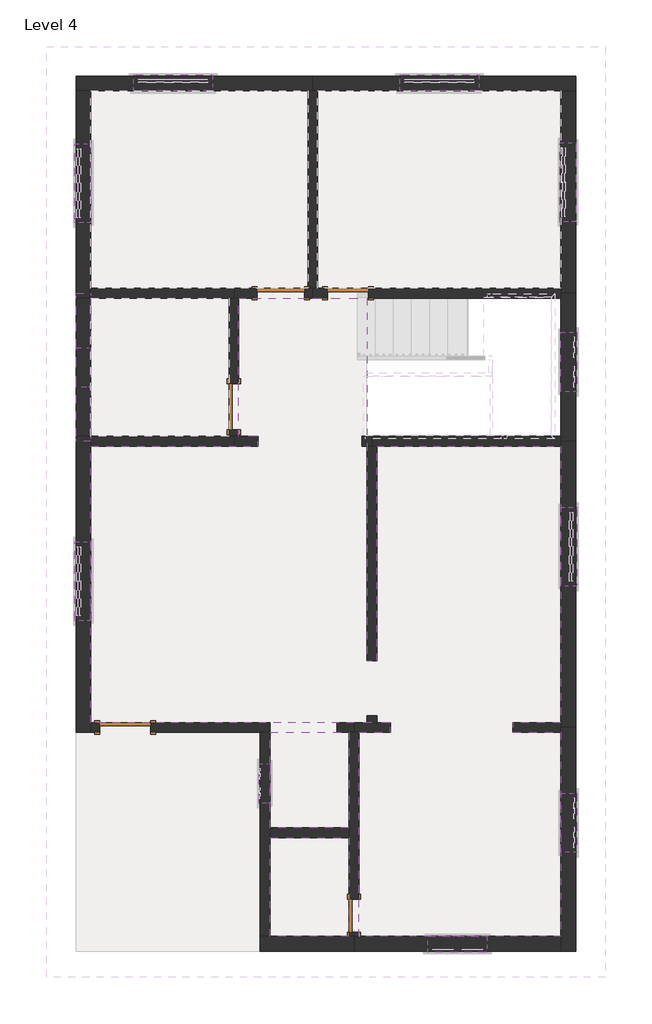
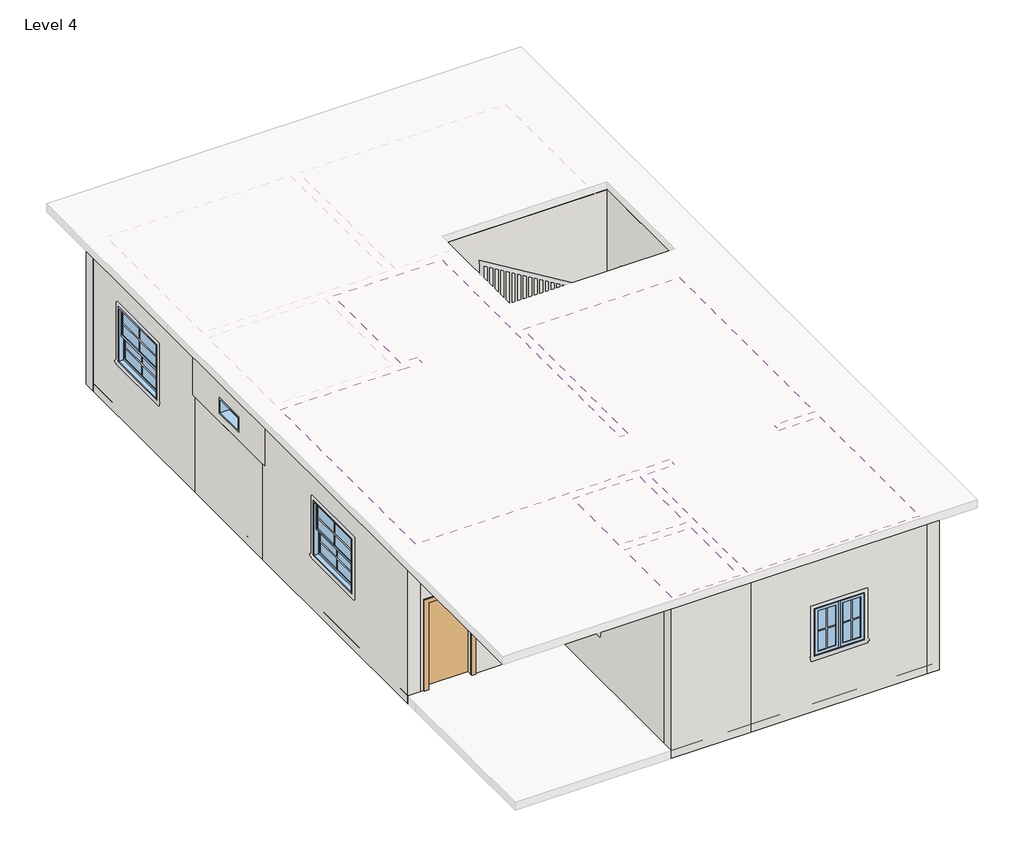
# One storey, part 1 of 2: 26 walls, 11 windows, 5 doors, 3 coverings.
"""IFC4 building model written with IfcOpenShell, lengths in millimetres."""

from ifc_helpers import new_model, si_unit, frame, origin, place, context, project, spatial, polyline, circle_curve, outline, extrude, faceted_brep, transform, mapped, element, save
from ifc_brep_helpers import plane_surface, revolved_surface, advanced_brep
from components import door_85c31a06, door_fe267433, door_77f51d0b, door_a6948854, door_ee35e093, fixed_2_8c8825d0, window_casement_double_2_fb285ced, window_casement_double_3_90de19e9, window_double_hung_4_eadb0177, window_double_hung_4_aab3aae7

model = new_model("IFC4")

# Units and contexts
model_context = context("Model", 3, world=origin())
ifc_project = project(units=[si_unit("LENGTHUNIT", "METRE", prefix="MILLI")], contexts=[model_context])

# Site, building, storey
site = spatial("IfcSite", under=ifc_project)
building = spatial("IfcBuilding", under=site)
storey = spatial("IfcBuildingStorey", under=building, Name="Level 4", Elevation=9601.2)

# Coverings
placement = place(None, origin())
element("IfcCovering", 1, ObjectType="2' x 4' ACT System", at=placement, inside=storey, context=model_context, shape_type="SweptSolid", body=[
    extrude(outline(polyline([(1592.635938, -3451.4142637), (1592.635938, -6601.0142637), (-1531.564062, -6601.0142637), (-1531.564062, -3451.4142637), (-1042.9877715, -3451.4142637), (-1042.9877715, -3299.0142637), (-1607.764062, -3299.0142637), (-5671.764062, -3299.0142637), (-5671.764062, 968.1857363), (-3538.164062, 968.1857363), (-3088.5741654, 968.1857363), (-3088.5741654, 1120.5857363), (-3385.764062, 1120.5857363), (-3385.764062, 3254.1857363), (-2242.764062, 3254.1857363), (-1404.564062, 3254.1857363), (-1404.564062, -2346.4297845), (-1252.164062, -2346.4297845), (-1252.164062, 968.1857363), (1592.635938, 968.1857363), (1592.635938, -3299.0142637), (852.655246, -3299.0142637), (852.655246, -3451.4142637), (1592.635938, -3451.4142637)])), frame((0.0, 0.0, 12649.2), z_axis=(0.0, 0.0, 1.0), x_axis=(1.0, 0.0, 0.0)), (0.0, 0.0, 1.0), 57.15),
])
element("IfcCovering", 2, ObjectType="2' x 4' ACT System", at=placement, inside=storey, context=model_context, shape_type="SweptSolid", body=[
    extrude(outline(polyline([(-2903.164062, -4924.6142637), (-2903.164062, -3451.4142637), (-1683.964062, -3451.4142637), (-1683.964062, -4924.6142637), (-2903.164062, -4924.6142637)])), frame((0.0, 0.0, 12649.2), z_axis=(0.0, 0.0, 1.0), x_axis=(1.0, 0.0, 0.0)), (0.0, 0.0, 1.0), 57.15),
])
element("IfcCovering", 3, ObjectType="2' x 4' ACT System", at=placement, inside=storey, context=model_context, shape_type="SweptSolid", body=[
    extrude(outline(polyline([(-2903.164062, -6601.0142637), (-2903.164062, -5077.0142637), (-1683.964062, -5077.0142637), (-1683.964062, -6601.0142637), (-2903.164062, -6601.0142637)])), frame((0.0, 0.0, 12649.2), z_axis=(0.0, 0.0, 1.0), x_axis=(1.0, 0.0, 0.0)), (0.0, 0.0, 1.0), 57.15),
])

# Doors
door_shape = door_85c31a06(model_context)
element("IfcDoor", 4, ObjectType="Single-Flush : 1'8\"", at=placement, inside=storey, context=model_context, shape_type="MappedRepresentation", body=[
    mapped(door_shape, transform((-1607.764062, -6283.5142637, 9753.6), x_axis=(0.0, -1.0, 0.0), y_axis=(1.0, 0.0, 0.0), z_axis=(0.0, 0.0, 1.0))),
])
door_2_shape = door_fe267433(model_context)
element("IfcDoor", 5, ObjectType="Single-Flush : 2'1\"", at=placement, inside=storey, context=model_context, shape_type="MappedRepresentation", body=[
    mapped(door_2_shape, transform((-1696.664062, 3330.3857363, 9753.6), x_axis=(-1.0, 0.0, 0.0), y_axis=(0.0, -1.0, 0.0), z_axis=(0.0, 0.0, 1.0))),
])
door_3_shape = door_77f51d0b(model_context)
element("IfcDoor", 6, ObjectType="Single-Flush : 2'4\"", at=placement, inside=storey, context=model_context, shape_type="MappedRepresentation", body=[
    mapped(door_3_shape, transform((-3461.964062, 1577.7857363, 9753.6), x_axis=(0.0, -1.0, 0.0), y_axis=(1.0, 0.0, 0.0), z_axis=(0.0, 0.0, 1.0))),
])
door_4_shape = door_a6948854(model_context)
element("IfcDoor", 7, ObjectType="Single-Flush : 2'5\"", at=placement, inside=storey, context=model_context, shape_type="MappedRepresentation", body=[
    mapped(door_4_shape, transform((-2738.064062, 3330.3857363, 9753.6), x_axis=(1.0, 0.0, 0.0), y_axis=(0.0, 1.0, 0.0), z_axis=(0.0, 0.0, 1.0))),
])
door_5_shape = door_ee35e093(model_context)
element("IfcDoor", 8, ObjectType="Single-Flush : 2'7\"", at=placement, inside=storey, context=model_context, shape_type="MappedRepresentation", body=[
    mapped(door_5_shape, transform((-5144.714062, -3375.2142637, 9753.6), x_axis=(-1.0, 0.0, 0.0), y_axis=(0.0, -1.0, 0.0), z_axis=(0.0, 0.0, 1.0))),
])

# Walls
element("IfcWall", 9, ObjectType="Generic - 6\"", at=placement, inside=storey, context=model_context, shape_type="Brep", body=[
    faceted_brep([(-2318.964062, 6454.5857363, 9753.6), (-2318.964062, 3406.5857363, 9753.6), (-2318.964062, 3406.5857363, 12954.0), (-2318.964062, 6454.5857363, 12954.0), (-2166.564062, 6454.5857363, 9753.6), (-2166.564062, 6454.5857363, 12954.0), (-2166.564062, 3406.5857363, 12954.0), (-2166.564062, 3406.5857363, 9753.6), (-2242.764062, 6454.5857363, 9753.6), (-2242.764062, 3406.5857363, 9753.6), (-2242.764062, 3406.5857363, 12954.0), (-2242.764062, 6454.5857363, 12954.0)], [[[0, 1, 2, 3]], [[4, 5, 6, 7]], [[1, 0, 8, 4, 7, 9]], [[3, 2, 10, 6, 5, 11]], [[0, 3, 11, 5, 4, 8]], [[2, 1, 9, 7, 6, 10]]]),
])
element("IfcWall", 10, ObjectType="Generic - 6\"", at=placement, inside=storey, context=model_context, shape_type="Brep", body=[
    faceted_brep([(-5671.764062, 3254.1857363, 12954.0), (-5671.764062, 3254.1857363, 11582.4), (-5671.764062, 3254.1857363, 9753.6), (-3538.164062, 3254.1857363, 9753.6), (-3461.964062, 3254.1857363, 9753.6), (-3461.964062, 3254.1857363, 12954.0), (-3538.164062, 3254.1857363, 12954.0), (-5671.764062, 3406.5857363, 9753.6), (-5671.764062, 3406.5857363, 12954.0), (-3461.964062, 3406.5857363, 12954.0), (-3461.964062, 3406.5857363, 9753.6), (-5671.764062, 3330.3857363, 12954.0)], [[[0, 1, 2, 3, 4, 5, 6]], [[7, 8, 9, 10]], [[4, 3, 2, 7, 10]], [[5, 4, 10, 9]], [[0, 6, 5, 9, 8, 11]], [[0, 11, 8, 7, 2, 1]]]),
])
element("IfcWall", 11, ObjectType="Generic - 6\"", at=placement, inside=storey, context=model_context, shape_type="Brep", body=[
    faceted_brep([(-5671.764062, 968.1857363, 12954.0), (-5671.764062, 968.1857363, 9753.6), (-3461.964062, 968.1857363, 9753.6), (-3461.964062, 968.1857363, 12954.0), (-5671.764062, 1120.5857363, 9753.6), (-5671.764062, 1120.5857363, 11582.4), (-5671.764062, 1120.5857363, 12954.0), (-3538.164062, 1120.5857363, 12954.0), (-3461.964062, 1120.5857363, 12954.0), (-3461.964062, 1120.5857363, 9753.6), (-3538.164062, 1120.5857363, 9753.6), (-5671.764062, 1044.3857363, 12954.0)], [[[0, 1, 2, 3]], [[4, 5, 6, 7, 8, 9, 10]], [[2, 1, 4, 10, 9]], [[3, 2, 9, 8]], [[0, 3, 8, 7, 6, 11]], [[0, 11, 6, 5, 4, 1]]]),
])
element("IfcWall", 12, ObjectType="Generic - 6\"", at=placement, inside=storey, context=model_context, shape_type="Brep", body=[
    faceted_brep([(-1404.564062, 968.1857363, 9753.6), (-1404.564062, -2346.4297845, 9753.6), (-1404.564062, -2346.4297845, 12217.4), (-1404.564062, -3197.4142637, 12217.4), (-1404.564062, -3197.4142637, 12039.6), (-1404.564062, -3197.4142637, 9753.6), (-1404.564062, -3299.0142637, 9753.6), (-1404.564062, -3299.0142637, 12954.0), (-1404.564062, 968.1857363, 12954.0), (-1252.164062, -2346.4297845, 9753.6), (-1252.164062, 968.1857363, 9753.6), (-1252.164062, 968.1857363, 12954.0), (-1252.164062, -3299.0142637, 12954.0), (-1252.164062, -3299.0142637, 9753.6), (-1252.164062, -3197.4142637, 9753.6), (-1252.164062, -3197.4142637, 12039.6), (-1252.164062, -3197.4142637, 12217.4), (-1252.164062, -2346.4297845, 12217.4), (-1328.364062, 968.1857363, 9753.6), (-1328.364062, 968.1857363, 12954.0)], [[[0, 1, 2, 3, 4, 5, 6, 7, 8]], [[9, 10, 11, 12, 13, 14, 15, 16, 17]], [[7, 6, 13, 12]], [[1, 0, 18, 10, 9]], [[8, 7, 12, 11, 19]], [[2, 1, 9, 17]], [[3, 2, 17, 16]], [[3, 16, 15, 14, 5, 4]], [[6, 5, 14, 13]], [[0, 8, 19, 11, 10, 18]]]),
])
element("IfcWall", 13, ObjectType="Generic - 6\"", at=placement, inside=storey, context=model_context, shape_type="Brep", body=[
    faceted_brep([(-2903.164062, -3451.4142637, 12039.6), (-1865.8319448, -3451.4142637, 12039.6), (-1865.8319448, -3451.4142637, 9753.6), (-1683.964062, -3451.4142637, 9753.6), (-1607.764062, -3451.4142637, 9753.6), (-1607.764062, -3451.4142637, 12954.0), (-1683.964062, -3451.4142637, 12954.0), (-2903.164062, -3451.4142637, 12954.0), (-3055.564062, -3451.4142637, 12954.0), (-5671.764062, -3451.4142637, 12954.0), (-5671.764062, -3451.4142637, 9753.6), (-5538.414062, -3451.4142637, 9753.6), (-5538.414062, -3451.4142637, 11582.4), (-4751.014062, -3451.4142637, 11582.4), (-4751.014062, -3451.4142637, 9753.6), (-3055.564062, -3451.4142637, 9753.6), (-2903.164062, -3451.4142637, 9753.6), (-1865.8319448, -3299.0142637, 12039.6), (-2903.164062, -3299.0142637, 12039.6), (-2903.164062, -3299.0142637, 9753.6), (-4751.014062, -3299.0142637, 9753.6), (-4751.014062, -3299.0142637, 11582.4), (-5538.414062, -3299.0142637, 11582.4), (-5538.414062, -3299.0142637, 9753.6), (-5671.764062, -3299.0142637, 9753.6), (-5671.764062, -3299.0142637, 12954.0), (-1607.764062, -3299.0142637, 12954.0), (-1607.764062, -3299.0142637, 9753.6), (-1865.8319448, -3299.0142637, 9753.6)], [[[0, 1, 2, 3, 4, 5, 6, 7, 8, 9, 10, 11, 12, 13, 14, 15, 16]], [[17, 18, 19, 20, 21, 22, 23, 24, 25, 26, 27, 28]], [[17, 1, 0, 18]], [[1, 17, 28, 2]], [[22, 12, 11, 23]], [[12, 22, 21, 13]], [[13, 21, 20, 14]], [[10, 24, 23, 11]], [[27, 4, 3, 2, 28]], [[19, 16, 15, 14, 20]], [[5, 4, 27, 26]], [[9, 8, 7, 6, 5, 26, 25]], [[10, 9, 25, 24]], [[18, 0, 16, 19]]]),
])
element("IfcWall", 14, ObjectType="Generic - 6\"", at=placement, inside=storey, context=model_context, shape_type="Brep", body=[
    faceted_brep([(-3055.564062, -3451.4142637, 9753.6), (-3055.564062, -6601.0142637, 9753.6), (-3055.564062, -6601.0142637, 12954.0), (-3055.564062, -3451.4142637, 12954.0), (-3055.564062, -3934.0142637, 11734.8), (-3055.564062, -4543.6142637, 11734.8), (-3055.564062, -4543.6142637, 10820.4), (-3055.564062, -3934.0142637, 10820.4), (-2903.164062, -3451.4142637, 9753.6), (-2903.164062, -3451.4142637, 12039.6), (-2903.164062, -3451.4142637, 12954.0), (-2903.164062, -4924.6142637, 12954.0), (-2903.164062, -5077.0142637, 12954.0), (-2903.164062, -6601.0142637, 12954.0), (-2903.164062, -6601.0142637, 9753.6), (-2903.164062, -5077.0142637, 9753.6), (-2903.164062, -4924.6142637, 9753.6), (-2903.164062, -3934.0142637, 11734.8), (-2903.164062, -3934.0142637, 10820.4), (-2903.164062, -4543.6142637, 10820.4), (-2903.164062, -4543.6142637, 11734.8)], [[[0, 1, 2, 3], [4, 5, 6, 7]], [[8, 9, 10, 11, 12, 13, 14, 15, 16], [17, 18, 19, 20]], [[1, 0, 8, 16, 15, 14]], [[3, 2, 13, 12, 11, 10]], [[2, 1, 14, 13]], [[18, 17, 4, 7]], [[19, 18, 7, 6]], [[20, 19, 6, 5]], [[17, 20, 5, 4]], [[0, 3, 10, 9, 8]]]),
])
element("IfcWall", 15, ObjectType="Generic - 6\"", at=placement, inside=storey, context=model_context, shape_type="Brep", body=[
    faceted_brep([(-1683.964062, -6601.0142637, 12954.0), (-1683.964062, -5077.0142637, 12954.0), (-1683.964062, -4924.6142637, 12954.0), (-1683.964062, -3451.4142637, 12954.0), (-1683.964062, -3451.4142637, 9753.6), (-1683.964062, -4924.6142637, 9753.6), (-1683.964062, -5077.0142637, 9753.6), (-1683.964062, -6029.5142637, 9753.6), (-1683.964062, -6029.5142637, 11582.4), (-1683.964062, -6537.5142637, 11582.4), (-1683.964062, -6537.5142637, 9753.6), (-1683.964062, -6601.0142637, 9753.6), (-1531.564062, -3451.4142637, 12954.0), (-1531.564062, -6601.0142637, 12954.0), (-1531.564062, -6601.0142637, 9753.6), (-1531.564062, -6537.5142637, 9753.6), (-1531.564062, -6537.5142637, 11582.4), (-1531.564062, -6029.5142637, 11582.4), (-1531.564062, -6029.5142637, 9753.6), (-1531.564062, -3451.4142637, 9753.6), (-1607.764062, -6601.0142637, 9753.6), (-1607.764062, -3451.4142637, 9753.6), (-1607.764062, -6601.0142637, 12954.0), (-1607.764062, -3451.4142637, 12954.0)], [[[0, 1, 2, 3, 4, 5, 6, 7, 8, 9, 10, 11]], [[12, 13, 14, 15, 16, 17, 18, 19]], [[14, 20, 11, 10, 15]], [[4, 21, 19, 18, 7, 6, 5]], [[3, 2, 1, 0, 22, 13, 12, 23]], [[9, 16, 15, 10]], [[16, 9, 8, 17]], [[17, 8, 7, 18]], [[0, 11, 20, 14, 13, 22]], [[4, 3, 23, 12, 19, 21]]]),
])
element("IfcWall", 16, ObjectType="Generic - 6\"", at=placement, inside=storey, context=model_context, shape_type="SweptSolid", body=[
    extrude(outline(polyline([(-1683.964062, -5077.0142637), (-2903.164062, -5077.0142637), (-2903.164062, -4924.6142637), (-1683.964062, -4924.6142637), (-1683.964062, -5077.0142637)])), frame((0.0, 0.0, 9753.6), z_axis=(0.0, 0.0, 1.0), x_axis=(1.0, 0.0, 0.0)), (0.0, 0.0, 1.0), 3200.4),
])
element("IfcWall", 17, ObjectType="Generic - 6\"", at=placement, inside=storey, context=model_context, shape_type="Brep", body=[
    faceted_brep([(-3538.164062, 1120.5857363, 12954.0), (-3538.164062, 3254.1857363, 12954.0), (-3538.164062, 3254.1857363, 9753.6), (-3538.164062, 1933.3857363, 9753.6), (-3538.164062, 1933.3857363, 11582.4), (-3538.164062, 1222.1857363, 11582.4), (-3538.164062, 1222.1857363, 9753.6), (-3538.164062, 1120.5857363, 9753.6), (-3385.764062, 3254.1857363, 12954.0), (-3385.764062, 1120.5857363, 12954.0), (-3385.764062, 1120.5857363, 9753.6), (-3385.764062, 1222.1857363, 9753.6), (-3385.764062, 1222.1857363, 11582.4), (-3385.764062, 1933.3857363, 11582.4), (-3385.764062, 1933.3857363, 9753.6), (-3385.764062, 3254.1857363, 9753.6), (-3461.964062, 3254.1857363, 9753.6), (-3461.964062, 1120.5857363, 9753.6), (-3461.964062, 1120.5857363, 12954.0), (-3461.964062, 3254.1857363, 12954.0)], [[[0, 1, 2, 3, 4, 5, 6, 7]], [[8, 9, 10, 11, 12, 13, 14, 15]], [[2, 16, 15, 14, 3]], [[10, 17, 7, 6, 11]], [[1, 0, 18, 9, 8, 19]], [[12, 5, 4, 13]], [[13, 4, 3, 14]], [[5, 12, 11, 6]], [[2, 1, 19, 8, 15, 16]], [[0, 7, 17, 10, 9, 18]]]),
])
element("IfcWall", 18, ObjectType="Generic - 6\"", at=placement, inside=storey, context=model_context, shape_type="Brep", body=[
    faceted_brep([(-2242.764062, 3254.1857363, 9753.6), (-2014.164062, 3254.1857363, 9753.6), (-2014.164062, 3254.1857363, 11582.4), (-1379.164062, 3254.1857363, 11582.4), (-1379.164062, 3254.1857363, 9753.6), (1592.635938, 3254.1857363, 9753.6), (1592.635938, 3254.1857363, 12954.0), (1563.3106034, 3254.1857363, 12954.0), (-2242.764062, 3254.1857363, 12954.0), (-2014.164062, 3406.5857363, 11582.4), (-2014.164062, 3406.5857363, 9753.6), (-2166.564062, 3406.5857363, 9753.6), (-2242.764062, 3406.5857363, 9753.6), (-2242.764062, 3406.5857363, 12954.0), (-2166.564062, 3406.5857363, 12954.0), (1592.635938, 3406.5857363, 12954.0), (1592.635938, 3406.5857363, 9753.6), (-1379.164062, 3406.5857363, 9753.6), (-1379.164062, 3406.5857363, 11582.4), (1592.635938, 3330.3857363, 9753.6), (1592.635938, 3330.3857363, 12954.0)], [[[0, 1, 2, 3, 4, 5, 6, 7, 8]], [[9, 10, 11, 12, 13, 14, 15, 16, 17, 18]], [[17, 16, 19, 5, 4]], [[12, 11, 10, 1, 0]], [[8, 7, 6, 20, 15, 14, 13]], [[0, 8, 13, 12]], [[4, 3, 18, 17]], [[3, 2, 9, 18]], [[2, 1, 10, 9]], [[5, 19, 16, 15, 20, 6]]]),
])
element("IfcWall", 19, ObjectType="Generic - 6\"", at=placement, inside=storey, context=model_context, shape_type="Brep", body=[
    faceted_brep([(1592.635938, 968.1857363, 9753.6), (1592.635938, 968.1857363, 12954.0), (-1252.164062, 968.1857363, 12954.0), (-1328.364062, 968.1857363, 12954.0), (-1328.364062, 968.1857363, 9753.6), (-1252.164062, 968.1857363, 9753.6), (1592.635938, 1120.5857363, 12954.0), (1592.635938, 1120.5857363, 9753.6), (-1328.364062, 1120.5857363, 9753.6), (-1328.364062, 1120.5857363, 12954.0), (1563.3106034, 1120.5857363, 12954.0), (1592.635938, 1044.3857363, 12954.0), (1592.635938, 1044.3857363, 9753.6)], [[[0, 1, 2, 3, 4, 5]], [[6, 7, 8, 9, 10]], [[3, 2, 1, 11, 6, 10, 9]], [[0, 5, 4, 8, 7, 12]], [[3, 9, 8, 4]], [[0, 12, 7, 6, 11, 1]]]),
])
element("IfcWall", 20, ObjectType="Generic - 6\"", at=placement, inside=storey, context=model_context, shape_type="AdvancedBrep", body=[
    advanced_brep(
    [(1592.635938, -3451.4142637, 12954.0), (-1531.564062, -3451.4142637, 12954.0), (-1607.764062, -3451.4142637, 12954.0), (-1607.764062, -3451.4142637, 9753.6), (-1531.564062, -3451.4142637, 9753.6), (-1042.9877715, -3451.4142637, 9753.6), (-1042.9877715, -3451.4142637, 12039.6), (-909.3649468, -3451.4142637, 12039.6), (732.5205767, -3451.4142637, 12039.6), (852.655246, -3451.4142637, 12039.6), (852.655246, -3451.4142637, 9753.6), (1592.635938, -3451.4142637, 9753.6), (-1607.764062, -3299.0142637, 12954.0), (-1404.564062, -3299.0142637, 12954.0), (-1252.164062, -3299.0142637, 12954.0), (1592.635938, -3299.0142637, 12954.0), (1592.635938, -3299.0142637, 9753.6), (852.655246, -3299.0142637, 9753.6), (852.655246, -3299.0142637, 12039.6), (732.5205767, -3299.0142637, 12039.6), (-909.3649468, -3299.0142637, 12039.6), (-1042.9877715, -3299.0142637, 12039.6), (-1042.9877715, -3299.0142637, 9753.6), (-1252.164062, -3299.0142637, 9753.6), (-1404.564062, -3299.0142637, 9753.6), (-1607.764062, -3299.0142637, 9753.6), (1592.635938, -3375.2142637, 12954.0), (1592.635938, -3375.2142637, 9753.6)],
    [
        (0, 1),
        (1, 2),
        (2, 3),
        (3, 4),
        (4, 5),
        (5, 6),
        (6, 7),
        (7, 8, circle_curve(frame((-88.4221851, -3451.4142637, 11503.8141821), z_axis=(0.0, 1.0, 0.0), x_axis=(-1.0, 0.0, 0.0)), 980.3129402)),
        (8, 9),
        (9, 10),
        (10, 11),
        (11, 0),
        (12, 13),
        (13, 14),
        (14, 15),
        (15, 16),
        (16, 17),
        (17, 18),
        (18, 19),
        (19, 20, circle_curve(frame((-88.4221851, -3299.0142637, 11503.8141821), z_axis=(0.0, -1.0, 0.0), x_axis=(-1.0, 0.0, 0.0)), 980.3129402)),
        (20, 21),
        (21, 22),
        (22, 23),
        (23, 24),
        (24, 25),
        (25, 12),
        (0, 26),
        (26, 15),
        (12, 2),
        (9, 18),
        (17, 10),
        (5, 22),
        (21, 6),
        (7, 20),
        (19, 8),
        (3, 25),
        (16, 27),
        (27, 11),
    ],
    [
        plane_surface(frame((1706.935938, -3451.4142637, 12954.0), z_axis=(0.0, -1.0, 0.0), x_axis=(-1.0, 0.0, 0.0))),
        plane_surface(frame((1706.935938, -3299.0142637, 12954.0), z_axis=(0.0, 1.0, 0.0), x_axis=(1.0, 0.0, 0.0))),
        plane_surface(frame((1706.935938, -3451.4142637, 12954.0), z_axis=(0.0, 0.0, 1.0), x_axis=(0.0, 1.0, 0.0))),
        plane_surface(frame((852.655246, -3451.4142637, 11778.380621), z_axis=(-1.0, 0.0, 0.0), x_axis=(0.0, 1.0, 0.0))),
        plane_surface(frame((-1042.9877715, -3451.4142637, 10089.1784957), z_axis=(1.0, 0.0, 0.0), x_axis=(0.0, 1.0, 0.0))),
        revolved_surface(polyline([(-1068.7351253, -3299.0142637, 11503.8141821), (-1068.7351253, -3451.4142637, 11503.8141821)]), (-88.4221851, -3299.0142637, 11503.8141821), (0.0, 1.0, 0.0)),
        plane_surface(frame((-1607.764062, -3451.4142637, 9753.6), z_axis=(0.0, 0.0, -1.0), x_axis=(0.0, 1.0, 0.0))),
        plane_surface(frame((456.9071606, -3451.4142637, 9753.6), z_axis=(0.0, 0.0, -1.0), x_axis=(0.0, 1.0, 0.0))),
        plane_surface(frame((-1607.764062, -3451.4142637, 12954.0), z_axis=(-1.0, 0.0, 0.0), x_axis=(0.0, 1.0, 0.0))),
        plane_surface(frame((1592.635938, 6454.5857363, 9753.6), z_axis=(1.0, 0.0, 0.0), x_axis=(0.0, -1.0, 0.0))),
        plane_surface(frame((-1042.9877715, -3299.0142637, 12039.6), z_axis=(0.0, 0.0, -1.0), x_axis=(-1.0, 0.0, 0.0))),
    ],
    [
        (0, [[1, 2, 3, 4, 5, 6, 7, 8, 9, 10, 11, 12]]),
        (1, [[13, 14, 15, 16, 17, 18, 19, 20, 21, 22, 23, 24, 25, 26]]),
        (2, [[-2, -1, 27, 28, -15, -14, -13, 29]]),
        (3, [[30, -18, 31, -10]]),
        (4, [[32, -22, 33, -6]]),
        (5, [[-8, 34, -20, 35]]),
        (6, [[36, -25, -24, -23, -32, -5, -4]]),
        (7, [[37, 38, -11, -31, -17]]),
        (8, [[-3, -29, -26, -36]]),
        (9, [[-12, -38, -37, -16, -28, -27]]),
        (10, [[-33, -21, -34, -7]]),
        (10, [[-30, -9, -35, -19]]),
    ],
),
])
element("IfcWall", 21, ObjectType="Generic - 6\"", at=placement, inside=storey, context=model_context, shape_type="Brep", body=[
    faceted_brep([(-2369.764062, 3254.1857363, 11582.4), (-2369.764062, 3254.1857363, 9753.6), (-2242.764062, 3254.1857363, 9753.6), (-2242.764062, 3254.1857363, 12954.0), (-3385.764062, 3254.1857363, 12954.0), (-3461.964062, 3254.1857363, 12954.0), (-3461.964062, 3254.1857363, 9753.6), (-3385.764062, 3254.1857363, 9753.6), (-3106.364062, 3254.1857363, 9753.6), (-3106.364062, 3254.1857363, 11582.4), (-2242.764062, 3406.5857363, 9753.6), (-2318.964062, 3406.5857363, 9753.6), (-2369.764062, 3406.5857363, 9753.6), (-2369.764062, 3406.5857363, 11582.4), (-3106.364062, 3406.5857363, 11582.4), (-3106.364062, 3406.5857363, 9753.6), (-3461.964062, 3406.5857363, 9753.6), (-3461.964062, 3406.5857363, 12954.0), (-2318.964062, 3406.5857363, 12954.0), (-2242.764062, 3406.5857363, 12954.0)], [[[0, 1, 2, 3, 4, 5, 6, 7, 8, 9]], [[10, 11, 12, 13, 14, 15, 16, 17, 18, 19]], [[2, 1, 12, 11, 10]], [[8, 7, 6, 16, 15]], [[3, 2, 10, 19]], [[5, 4, 3, 19, 18, 17]], [[6, 5, 17, 16]], [[15, 14, 9, 8]], [[14, 13, 0, 9]], [[13, 12, 1, 0]]]),
])
element("IfcWall", 22, ObjectType="Generic - 6\"", at=placement, inside=storey, context=model_context, shape_type="AdvancedBrep", body=[
    advanced_brep(
    [(-1328.364062, 968.1857363, 12954.0), (-1404.564062, 968.1857363, 12954.0), (-3461.964062, 968.1857363, 12954.0), (-3461.964062, 968.1857363, 9753.6), (-3088.5741654, 968.1857363, 9753.6), (-3088.5741654, 968.1857363, 12039.6), (-2990.069581, 968.1857363, 12039.6), (-1595.0493956, 968.1857363, 12039.6), (-1480.764062, 968.1857363, 12039.6), (-1480.764062, 968.1857363, 9753.6), (-1404.564062, 968.1857363, 9753.6), (-1328.364062, 968.1857363, 9753.6), (-3461.964062, 1120.5857363, 12954.0), (-3385.764062, 1120.5857363, 12954.0), (-1328.364062, 1120.5857363, 12954.0), (-1328.364062, 1120.5857363, 9753.6), (-1480.764062, 1120.5857363, 9753.6), (-1480.764062, 1120.5857363, 12039.6), (-1595.0493956, 1120.5857363, 12039.6), (-2990.069581, 1120.5857363, 12039.6), (-3088.5741654, 1120.5857363, 12039.6), (-3088.5741654, 1120.5857363, 9753.6), (-3385.764062, 1120.5857363, 9753.6), (-3461.964062, 1120.5857363, 9753.6)],
    [
        (0, 1),
        (1, 2),
        (2, 3),
        (3, 4),
        (4, 5),
        (5, 6),
        (6, 7, circle_curve(frame((-2292.5594883, 968.1857363, 11861.8), z_axis=(0.0, 1.0, 0.0), x_axis=(-1.0, 0.0, 0.0)), 719.8146771)),
        (7, 8),
        (8, 9),
        (9, 10),
        (10, 11),
        (11, 0),
        (12, 13),
        (13, 14),
        (14, 15),
        (15, 16),
        (16, 17),
        (17, 18),
        (18, 19, circle_curve(frame((-2292.5594883, 1120.5857363, 11861.8), z_axis=(0.0, -1.0, 0.0), x_axis=(-1.0, 0.0, 0.0)), 719.8146771)),
        (19, 20),
        (20, 21),
        (21, 22),
        (22, 23),
        (23, 12),
        (6, 19),
        (18, 7),
        (15, 11),
        (9, 16),
        (0, 14),
        (12, 2),
        (3, 23),
        (21, 4),
        (5, 20),
        (17, 8),
    ],
    [
        plane_surface(frame((-3012.3741654, 968.1857363, 11861.8), z_axis=(0.0, -1.0, 0.0), x_axis=(0.0, 0.0, 1.0))),
        plane_surface(frame((-3012.3741654, 1120.5857363, 11861.8), z_axis=(0.0, 1.0, 0.0), x_axis=(0.0, 0.0, -1.0))),
        revolved_surface(polyline([(-3012.3741654, 1120.5857363, 11861.8), (-3012.3741654, 968.1857363, 11861.8)]), (-2292.5594883, 1120.5857363, 11861.8), (0.0, 1.0, 0.0)),
        plane_surface(frame((-1572.7448112, 968.1857363, 9753.6), z_axis=(0.0, 0.0, -1.0), x_axis=(0.0, 1.0, 0.0))),
        plane_surface(frame((-1328.364062, 968.1857363, 12954.0), z_axis=(0.0, 0.0, 1.0), x_axis=(0.0, 1.0, 0.0))),
        plane_surface(frame((-3461.964062, 968.1857363, 9753.6), z_axis=(0.0, 0.0, -1.0), x_axis=(0.0, 1.0, 0.0))),
        plane_surface(frame((-1328.364062, 968.1857363, 9753.6), z_axis=(1.0, 0.0, 0.0), x_axis=(0.0, 1.0, 0.0))),
        plane_surface(frame((-3461.964062, 968.1857363, 12954.0), z_axis=(-1.0, 0.0, 0.0), x_axis=(0.0, 1.0, 0.0))),
        plane_surface(frame((-3088.5741654, 1120.5857363, 12039.6), z_axis=(0.0, 0.0, -1.0), x_axis=(-1.0, 0.0, 0.0))),
        plane_surface(frame((-3088.5741654, 1120.5857363, 12039.6), z_axis=(1.0, 0.0, 0.0), x_axis=(0.0, 0.0, -1.0))),
        plane_surface(frame((-1480.764062, 968.1857363, 12039.6), z_axis=(-1.0, 0.0, 0.0), x_axis=(0.0, 0.0, -1.0))),
    ],
    [
        (0, [[1, 2, 3, 4, 5, 6, 7, 8, 9, 10, 11, 12]]),
        (1, [[13, 14, 15, 16, 17, 18, 19, 20, 21, 22, 23, 24]]),
        (2, [[-7, 25, -19, 26]]),
        (3, [[27, -11, -10, 28, -16]]),
        (4, [[-2, -1, 29, -14, -13, 30]]),
        (5, [[31, -23, -22, 32, -4]]),
        (6, [[-12, -27, -15, -29]]),
        (7, [[-3, -30, -24, -31]]),
        (8, [[33, -20, -25, -6]]),
        (8, [[34, -8, -26, -18]]),
        (9, [[-33, -5, -32, -21]]),
        (10, [[-34, -17, -28, -9]]),
    ],
),
])
element("IfcWall", 23, ObjectType="Generic - 9\"", at=placement, inside=storey, context=model_context, shape_type="Brep", body=[
    faceted_brep([(-5900.364062, 6454.5857363, 9753.6), (-5671.764062, 6454.5857363, 9753.6), (-2318.964062, 6454.5857363, 9753.6), (-2242.764062, 6454.5857363, 9753.6), (-2242.764062, 6454.5857363, 12954.0), (-2318.964062, 6454.5857363, 12954.0), (-5671.764062, 6454.5857363, 12954.0), (-5900.364062, 6454.5857363, 12954.0), (-3792.164062, 6454.5857363, 11887.2), (-3792.164062, 6454.5857363, 10820.4), (-5011.364062, 6454.5857363, 10820.4), (-5011.364062, 6454.5857363, 11887.2), (-5900.364062, 6683.1857363, 9753.6), (-5900.364062, 6683.1857363, 12954.0), (-2242.764062, 6683.1857363, 12954.0), (-2242.764062, 6683.1857363, 9753.6), (-3792.164062, 6683.1857363, 11887.2), (-5011.364062, 6683.1857363, 11887.2), (-5011.364062, 6683.1857363, 10820.4), (-3792.164062, 6683.1857363, 10820.4)], [[[0, 1, 2, 3, 4, 5, 6, 7], [8, 9, 10, 11]], [[12, 13, 14, 15], [16, 17, 18, 19]], [[3, 2, 1, 0, 12, 15]], [[4, 3, 15, 14]], [[7, 6, 5, 4, 14, 13]], [[0, 7, 13, 12]], [[9, 8, 16, 19]], [[10, 9, 19, 18]], [[11, 10, 18, 17]], [[8, 11, 17, 16]]]),
])
element("IfcWall", 24, ObjectType="Generic - 9\"", at=placement, inside=storey, context=model_context, shape_type="Brep", body=[
    faceted_brep([(1592.635938, 6454.5857363, 9753.6), (1592.635938, 3406.5857363, 9753.6), (1592.635938, 3330.3857363, 9753.6), (1592.635938, 3330.3857363, 12954.0), (1592.635938, 3362.5242824, 12954.0), (1592.635938, 3406.5857363, 12954.0), (1592.635938, 6454.5857363, 12954.0), (1592.635938, 5654.4857363, 11887.2), (1592.635938, 4435.2857363, 11887.2), (1592.635938, 4435.2857363, 10820.4), (1592.635938, 5654.4857363, 10820.4), (1821.235938, 6454.5857363, 9753.6), (1821.235938, 6454.5857363, 12954.0), (1821.235938, 3330.3857363, 12954.0), (1821.235938, 3330.3857363, 9753.6), (1821.235938, 5654.4857363, 11887.2), (1821.235938, 5654.4857363, 10820.4), (1821.235938, 4435.2857363, 10820.4), (1821.235938, 4435.2857363, 11887.2)], [[[0, 1, 2, 3, 4, 5, 6], [7, 8, 9, 10]], [[11, 12, 13, 14], [15, 16, 17, 18]], [[2, 1, 0, 11, 14]], [[6, 5, 4, 3, 13, 12]], [[0, 6, 12, 11]], [[16, 15, 7, 10]], [[17, 16, 10, 9]], [[18, 17, 9, 8]], [[15, 18, 8, 7]], [[2, 14, 13, 3]]]),
])
element("IfcWall", 25, ObjectType="Generic - 9\"", at=placement, inside=storey, context=model_context, shape_type="Brep", body=[
    faceted_brep([(1592.635938, -6601.0142637, 9753.6), (-1531.564062, -6601.0142637, 9753.6), (-1607.764062, -6601.0142637, 9753.6), (-1607.764062, -6601.0142637, 12954.0), (-1531.564062, -6601.0142637, 12954.0), (1592.635938, -6601.0142637, 12954.0), (-464.764062, -6601.0142637, 11734.8), (-464.764062, -6601.0142637, 10820.4), (449.635938, -6601.0142637, 10820.4), (449.635938, -6601.0142637, 11734.8), (1592.635938, -6829.6142637, 9753.6), (1592.635938, -6829.6142637, 12954.0), (-1607.764062, -6829.6142637, 12954.0), (-1607.764062, -6829.6142637, 9753.6), (-464.764062, -6829.6142637, 11734.8), (449.635938, -6829.6142637, 11734.8), (449.635938, -6829.6142637, 10820.4), (-464.764062, -6829.6142637, 10820.4)], [[[0, 1, 2, 3, 4, 5], [6, 7, 8, 9]], [[10, 11, 12, 13], [14, 15, 16, 17]], [[2, 1, 0, 10, 13]], [[3, 2, 13, 12]], [[5, 4, 3, 12, 11]], [[0, 5, 11, 10]], [[7, 6, 14, 17]], [[8, 7, 17, 16]], [[9, 8, 16, 15]], [[6, 9, 15, 14]]]),
])
element("IfcWall", 26, ObjectType="Generic - 9\"", at=placement, inside=storey, context=model_context, shape_type="Brep", body=[
    faceted_brep([(-5900.364062, 6454.5857363, 9753.6), (-5900.364062, 3254.1857363, 9753.6), (-5900.364062, 3254.1857363, 11582.4), (-5900.364062, 3330.3857363, 11582.4), (-5900.364062, 3330.3857363, 12954.0), (-5900.364062, 6454.5857363, 12954.0), (-5900.364062, 4422.5857363, 11887.2), (-5900.364062, 4422.5857363, 10820.4), (-5900.364062, 5641.7857363, 10820.4), (-5900.364062, 5641.7857363, 11887.2), (-5671.764062, 6454.5857363, 9753.6), (-5671.764062, 6454.5857363, 12954.0), (-5671.764062, 3406.5857363, 12954.0), (-5671.764062, 3330.3857363, 12954.0), (-5671.764062, 3330.3857363, 11582.4), (-5671.764062, 3254.1857363, 11582.4), (-5671.764062, 3254.1857363, 9753.6), (-5671.764062, 3406.5857363, 9753.6), (-5671.764062, 4422.5857363, 11887.2), (-5671.764062, 5641.7857363, 11887.2), (-5671.764062, 5641.7857363, 10820.4), (-5671.764062, 4422.5857363, 10820.4)], [[[0, 1, 2, 3, 4, 5], [6, 7, 8, 9]], [[10, 11, 12, 13, 14, 15, 16, 17], [18, 19, 20, 21]], [[1, 0, 10, 17, 16]], [[5, 4, 13, 12, 11]], [[0, 5, 11, 10]], [[7, 6, 18, 21]], [[8, 7, 21, 20]], [[9, 8, 20, 19]], [[6, 9, 19, 18]], [[4, 3, 14, 13]], [[14, 3, 2, 15]], [[2, 1, 16, 15]]]),
])
element("IfcWall", 27, ObjectType="Generic - 9\"", at=placement, inside=storey, context=model_context, shape_type="Brep", body=[
    faceted_brep([(-2242.764062, 6454.5857363, 9753.6), (-2166.564062, 6454.5857363, 9753.6), (1592.635938, 6454.5857363, 9753.6), (1821.235938, 6454.5857363, 9753.6), (1821.235938, 6454.5857363, 12954.0), (1592.635938, 6454.5857363, 12954.0), (-2166.564062, 6454.5857363, 12954.0), (-2242.764062, 6454.5857363, 12954.0), (322.635938, 6454.5857363, 11887.2), (322.635938, 6454.5857363, 10820.4), (-896.564062, 6454.5857363, 10820.4), (-896.564062, 6454.5857363, 11887.2), (-2242.764062, 6683.1857363, 9753.6), (-2242.764062, 6683.1857363, 12954.0), (1821.235938, 6683.1857363, 12954.0), (1821.235938, 6683.1857363, 9753.6), (322.635938, 6683.1857363, 11887.2), (-896.564062, 6683.1857363, 11887.2), (-896.564062, 6683.1857363, 10820.4), (322.635938, 6683.1857363, 10820.4)], [[[0, 1, 2, 3, 4, 5, 6, 7], [8, 9, 10, 11]], [[12, 13, 14, 15], [16, 17, 18, 19]], [[3, 2, 1, 0, 12, 15]], [[7, 6, 5, 4, 14, 13]], [[0, 7, 13, 12]], [[4, 3, 15, 14]], [[8, 11, 17, 16]], [[11, 10, 18, 17]], [[10, 9, 19, 18]], [[9, 8, 16, 19]]]),
])
element("IfcWall", 28, ObjectType="Generic - 9\"", at=placement, inside=storey, context=model_context, shape_type="Brep", body=[
    faceted_brep([(-1607.764062, -6601.0142637, 9753.6), (-1683.964062, -6601.0142637, 9753.6), (-2903.164062, -6601.0142637, 9753.6), (-3055.564062, -6601.0142637, 9753.6), (-3055.564062, -6601.0142637, 12954.0), (-2903.164062, -6601.0142637, 12954.0), (-1683.964062, -6601.0142637, 12954.0), (-1607.764062, -6601.0142637, 12954.0), (-1607.764062, -6829.6142637, 9753.6), (-1607.764062, -6829.6142637, 12954.0), (-3055.564062, -6829.6142637, 12954.0), (-3055.564062, -6829.6142637, 9753.6)], [[[0, 1, 2, 3, 4, 5, 6, 7]], [[8, 9, 10, 11]], [[3, 2, 1, 0, 8, 11]], [[7, 6, 5, 4, 10, 9]], [[0, 7, 9, 8]], [[4, 3, 11, 10]]]),
])
element("IfcWall", 29, ObjectType="Generic - 9\"", at=placement, inside=storey, context=model_context, shape_type="Brep", body=[
    faceted_brep([(1592.635938, 3330.3857363, 12954.0), (1592.635938, 3330.3857363, 9753.6), (1592.635938, 3254.1857363, 9753.6), (1592.635938, 1120.5857363, 9753.6), (1592.635938, 1044.3857363, 9753.6), (1592.635938, 1044.3857363, 12954.0), (1592.635938, 1120.5857363, 12954.0), (1592.635938, 1152.7242824, 12954.0), (1592.635938, 3210.1242824, 12954.0), (1592.635938, 3254.1857363, 12954.0), (1592.635938, 1812.7357363, 11734.8), (1592.635938, 1812.7357363, 10820.4), (1592.635938, 2727.1357363, 10820.4), (1592.635938, 2727.1357363, 11734.8), (1821.235938, 3330.3857363, 9753.6), (1821.235938, 3330.3857363, 12954.0), (1821.235938, 1044.3857363, 12954.0), (1821.235938, 1044.3857363, 9753.6), (1821.235938, 1812.7357363, 11734.8), (1821.235938, 2727.1357363, 11734.8), (1821.235938, 2727.1357363, 10820.4), (1821.235938, 1812.7357363, 10820.4)], [[[0, 1, 2, 3, 4, 5, 6, 7, 8, 9], [10, 11, 12, 13]], [[14, 15, 16, 17], [18, 19, 20, 21]], [[4, 3, 2, 1, 14, 17]], [[0, 9, 8, 7, 6, 5, 16, 15]], [[10, 13, 19, 18]], [[13, 12, 20, 19]], [[12, 11, 21, 20]], [[11, 10, 18, 21]], [[0, 15, 14, 1]], [[4, 17, 16, 5]]]),
])
element("IfcWall", 30, ObjectType="Generic - 9\"", at=placement, inside=storey, context=model_context, shape_type="Brep", body=[
    faceted_brep([(1592.635938, 1044.3857363, 12954.0), (1592.635938, 1044.3857363, 9753.6), (1592.635938, 968.1857363, 9753.6), (1592.635938, -3299.0142637, 9753.6), (1592.635938, -3375.2142637, 9753.6), (1592.635938, -3375.2142637, 12954.0), (1592.635938, -3299.0142637, 12954.0), (1592.635938, 968.1857363, 12954.0), (1592.635938, 1000.3242824, 12954.0), (1592.635938, 28.3857363, 11887.2), (1592.635938, -1190.8142637, 11887.2), (1592.635938, -1190.8142637, 10820.4), (1592.635938, 28.3857363, 10820.4), (1821.235938, 1044.3857363, 9753.6), (1821.235938, 1044.3857363, 12954.0), (1821.235938, -3375.2142637, 12954.0), (1821.235938, -3375.2142637, 9753.6), (1821.235938, 28.3857363, 11887.2), (1821.235938, 28.3857363, 10820.4), (1821.235938, -1190.8142637, 10820.4), (1821.235938, -1190.8142637, 11887.2)], [[[0, 1, 2, 3, 4, 5, 6, 7, 8], [9, 10, 11, 12]], [[13, 14, 15, 16], [17, 18, 19, 20]], [[4, 3, 2, 1, 13, 16]], [[5, 4, 16, 15]], [[0, 8, 7, 6, 5, 15, 14]], [[17, 20, 10, 9]], [[20, 19, 11, 10]], [[19, 18, 12, 11]], [[18, 17, 9, 12]], [[0, 14, 13, 1]]]),
])
element("IfcWall", 31, ObjectType="Generic - 9\"", at=placement, inside=storey, context=model_context, shape_type="Brep", body=[
    faceted_brep([(1592.635938, -3375.2142637, 9753.6), (1592.635938, -3451.4142637, 9753.6), (1592.635938, -6601.0142637, 9753.6), (1592.635938, -6829.6142637, 9753.6), (1592.635938, -6829.6142637, 12954.0), (1592.635938, -6601.0142637, 12954.0), (1592.635938, -3451.4142637, 12954.0), (1592.635938, -3375.2142637, 12954.0), (1592.635938, -5305.6142637, 11734.8), (1592.635938, -5305.6142637, 10820.4), (1592.635938, -4391.2142637, 10820.4), (1592.635938, -4391.2142637, 11734.8), (1821.235938, -3375.2142637, 9753.6), (1821.235938, -3375.2142637, 12954.0), (1821.235938, -6829.6142637, 12954.0), (1821.235938, -6829.6142637, 9753.6), (1821.235938, -5305.6142637, 11734.8), (1821.235938, -4391.2142637, 11734.8), (1821.235938, -4391.2142637, 10820.4), (1821.235938, -5305.6142637, 10820.4)], [[[0, 1, 2, 3, 4, 5, 6, 7], [8, 9, 10, 11]], [[12, 13, 14, 15], [16, 17, 18, 19]], [[3, 2, 1, 0, 12, 15]], [[7, 6, 5, 4, 14, 13]], [[0, 7, 13, 12]], [[4, 3, 15, 14]], [[8, 11, 17, 16]], [[11, 10, 18, 17]], [[10, 9, 19, 18]], [[9, 8, 16, 19]]]),
])
element("IfcWall", 32, ObjectType="Generic - 9\"", at=placement, inside=storey, context=model_context, shape_type="Brep", body=[
    faceted_brep([(-5900.364062, 1120.5857363, 9753.6), (-5900.364062, -3451.4142637, 9753.6), (-5900.364062, -3451.4142637, 12954.0), (-5900.364062, 1044.3857363, 12954.0), (-5900.364062, 1044.3857363, 11582.4), (-5900.364062, 1120.5857363, 11582.4), (-5900.364062, -1724.2142637, 11887.2), (-5900.364062, -1724.2142637, 10820.4), (-5900.364062, -505.0142637, 10820.4), (-5900.364062, -505.0142637, 11887.2), (-5671.764062, 1120.5857363, 9753.6), (-5671.764062, 1120.5857363, 11582.4), (-5671.764062, 1044.3857363, 11582.4), (-5671.764062, 1044.3857363, 12954.0), (-5671.764062, 968.1857363, 12954.0), (-5671.764062, -3299.0142637, 12954.0), (-5671.764062, -3451.4142637, 12954.0), (-5671.764062, -3451.4142637, 9753.6), (-5671.764062, -3299.0142637, 9753.6), (-5671.764062, 968.1857363, 9753.6), (-5671.764062, -1724.2142637, 11887.2), (-5671.764062, -505.0142637, 11887.2), (-5671.764062, -505.0142637, 10820.4), (-5671.764062, -1724.2142637, 10820.4)], [[[0, 1, 2, 3, 4, 5], [6, 7, 8, 9]], [[10, 11, 12, 13, 14, 15, 16, 17, 18, 19], [20, 21, 22, 23]], [[1, 0, 10, 19, 18, 17]], [[3, 2, 16, 15, 14, 13]], [[2, 1, 17, 16]], [[6, 9, 21, 20]], [[9, 8, 22, 21]], [[8, 7, 23, 22]], [[7, 6, 20, 23]], [[4, 3, 13, 12]], [[4, 12, 11, 5]], [[0, 5, 11, 10]]]),
])
element("IfcWall", 33, ObjectType="Generic - 9\"", at=placement, inside=storey, context=model_context, shape_type="Brep", body=[
    faceted_brep([(-5900.364062, 3330.3857363, 11582.4), (-5900.364062, 3254.1857363, 11582.4), (-5900.364062, 1120.5857363, 11582.4), (-5900.364062, 1044.3857363, 11582.4), (-5900.364062, 1044.3857363, 12954.0), (-5900.364062, 3330.3857363, 12954.0), (-5900.364062, 1882.5857363, 12039.6), (-5900.364062, 1882.5857363, 11734.8), (-5900.364062, 2492.1857363, 11734.8), (-5900.364062, 2492.1857363, 12039.6), (-5671.764062, 3330.3857363, 11582.4), (-5671.764062, 3330.3857363, 12954.0), (-5671.764062, 3254.1857363, 12954.0), (-5671.764062, 1120.5857363, 12954.0), (-5671.764062, 1044.3857363, 12954.0), (-5671.764062, 1044.3857363, 11582.4), (-5671.764062, 1120.5857363, 11582.4), (-5671.764062, 3254.1857363, 11582.4), (-5671.764062, 1882.5857363, 12039.6), (-5671.764062, 2492.1857363, 12039.6), (-5671.764062, 2492.1857363, 11734.8), (-5671.764062, 1882.5857363, 11734.8)], [[[0, 1, 2, 3, 4, 5], [6, 7, 8, 9]], [[10, 11, 12, 13, 14, 15, 16, 17], [18, 19, 20, 21]], [[3, 2, 1, 0, 10, 17, 16, 15]], [[4, 3, 15, 14]], [[5, 4, 14, 13, 12, 11]], [[0, 5, 11, 10]], [[6, 9, 19, 18]], [[9, 8, 20, 19]], [[8, 7, 21, 20]], [[7, 6, 18, 21]]]),
])
element("IfcWall", 34, ObjectType="Generic - 9\"", at=placement, inside=storey, context=model_context, shape_type="SweptSolid", body=[
    extrude(outline(polyline([(-5900.364062, 1120.5857363), (-5900.364062, 3254.1857363), (-5671.764062, 3254.1857363), (-5671.764062, 1120.5857363), (-5900.364062, 1120.5857363)])), frame((0.0, 0.0, 9753.6), z_axis=(0.0, 0.0, 1.0), x_axis=(1.0, 0.0, 0.0)), (0.0, 0.0, 1.0), 1828.8),
])

# Windows
fixed_2_shape = fixed_2_8c8825d0(model_context)
element("IfcWindow", 35, ObjectType="Fixed : 2'", at=placement, inside=storey, context=model_context, shape_type="MappedRepresentation", body=[
    mapped(fixed_2_shape, transform((-5786.064062, 2149.2857363, 10820.4), x_axis=(0.0, -1.0, 0.0), y_axis=(1.0, 0.0, 0.0), z_axis=(0.0, 0.0, 1.0))),
])
window_casement_double_2_shape = window_casement_double_2_fb285ced(model_context)
element("IfcWindow", 36, ObjectType="Window-Casement-Double : 2'", at=placement, inside=storey, context=model_context, shape_type="MappedRepresentation", body=[
    mapped(window_casement_double_2_shape, transform((-2979.364062, -4238.8142637, 9906.0), x_axis=(0.0, 1.0, 0.0), y_axis=(-1.0, 0.0, 0.0), z_axis=(0.0, 0.0, 1.0))),
])
window_casement_double_3_shape = window_casement_double_3_90de19e9(model_context)
element("IfcWindow", 37, ObjectType="Window-Casement-Double : 3'", at=placement, inside=storey, context=model_context, shape_type="MappedRepresentation", body=[
    mapped(window_casement_double_3_shape, transform((1706.935938, -4848.4142637, 9906.0), x_axis=(0.0, -1.0, 0.0), y_axis=(1.0, 0.0, 0.0), z_axis=(0.0, 0.0, 1.0))),
])
element("IfcWindow", 38, ObjectType="Window-Casement-Double : 3'", at=placement, inside=storey, context=model_context, shape_type="MappedRepresentation", body=[
    mapped(window_casement_double_3_shape, transform((-7.564062, -6715.3142637, 9906.0), x_axis=(-1.0, 0.0, 0.0), y_axis=(0.0, -1.0, 0.0), z_axis=(0.0, 0.0, 1.0))),
])
element("IfcWindow", 39, ObjectType="Window-Casement-Double : 3'", at=placement, inside=storey, context=model_context, shape_type="MappedRepresentation", body=[
    mapped(window_casement_double_3_shape, transform((1706.935938, 2269.9357363, 9906.0), x_axis=(0.0, -1.0, 0.0), y_axis=(1.0, 0.0, 0.0), z_axis=(0.0, 0.0, 1.0))),
])
window_double_hung_4_shape = window_double_hung_4_eadb0177(model_context)
element("IfcWindow", 40, ObjectType="Window-Double-Hung : 4'", at=placement, inside=storey, context=model_context, shape_type="MappedRepresentation", body=[
    mapped(window_double_hung_4_shape, transform((-5786.064062, 5032.1857363, 9906.0), x_axis=(0.0, 1.0, 0.0), y_axis=(-1.0, 0.0, 0.0), z_axis=(0.0, 0.0, 1.0))),
])
element("IfcWindow", 41, ObjectType="Window-Double-Hung : 4'", at=placement, inside=storey, context=model_context, shape_type="MappedRepresentation", body=[
    mapped(window_double_hung_4_shape, transform((1706.935938, -581.2142637, 9906.0), x_axis=(0.0, -1.0, 0.0), y_axis=(1.0, 0.0, 0.0), z_axis=(0.0, 0.0, 1.0))),
])
element("IfcWindow", 42, ObjectType="Window-Double-Hung : 4'", at=placement, inside=storey, context=model_context, shape_type="MappedRepresentation", body=[
    mapped(window_double_hung_4_shape, transform((-5786.064062, -1114.6142637, 9906.0), x_axis=(0.0, 1.0, 0.0), y_axis=(-1.0, 0.0, 0.0), z_axis=(0.0, 0.0, 1.0))),
])
window_double_hung_4_2_shape = window_double_hung_4_aab3aae7(model_context)
element("IfcWindow", 43, ObjectType="Window-Double-Hung : 4'", at=placement, inside=storey, context=model_context, shape_type="MappedRepresentation", body=[
    mapped(window_double_hung_4_2_shape, transform((-4401.764062, 6568.8857363, 9906.0), x_axis=(-1.0, 0.0, 0.0), y_axis=(0.0, -1.0, 0.0), z_axis=(0.0, 0.0, 1.0))),
])
element("IfcWindow", 44, ObjectType="Window-Double-Hung : 4'", at=placement, inside=storey, context=model_context, shape_type="MappedRepresentation", body=[
    mapped(window_double_hung_4_2_shape, transform((-286.964062, 6568.8857363, 9906.0), x_axis=(-1.0, 0.0, 0.0), y_axis=(0.0, -1.0, 0.0), z_axis=(0.0, 0.0, 1.0))),
])
element("IfcWindow", 45, ObjectType="Window-Double-Hung : 4'", at=placement, inside=storey, context=model_context, shape_type="MappedRepresentation", body=[
    mapped(window_double_hung_4_2_shape, transform((1706.935938, 5044.8857363, 9906.0), x_axis=(0.0, -1.0, 0.0), y_axis=(1.0, 0.0, 0.0), z_axis=(0.0, 0.0, 1.0))),
])

save(model, "model.ifc")

# Revit data of these elements
# Type "2' x 4' ACT System"
#   Assembly Code = "C3030210"
#   built-in parameter 1002203 = 1 (stored number, unit not read)
#   built-in parameter 1002202 = 1 (stored number, unit not read)
#   Layers, outside or top first: 0' - 1 5/8" "Default" (function 1); 0' - 0 5/8" "Acoustic Ceiling Tile 24 x 48" (function 5)
# Type "Single-Flush : 1'8\""
#   Type Mark = "11"
#   Construction Type Id = "MDOOR"
#   Assembly Code = "C1020"
#   Analytic Construction = "Metal"
#   Thickness = 0' - 2"
#   Heat Transfer Coefficient (U) = 0.651978 BTU/(h·ft²·°F)
#   Height = 6' - 0"
#   Trim Projection Ext = 0' - 1"
#   Trim Projection Int = 0' - 1"
#   Trim Width = 0' - 3"
#   Width = 1' - 8"
#   Define Thermal Properties by = 1
#   Door Material = Door - Panel
#   Frame Material = Door - Frame
#   Visual Light Transmittance = 0
#   Solar Heat Gain Coefficient = 0
#   Function = (empty or 0)
#   Wall Closure = (empty or 0)
# Type "Single-Flush : 2'1\""
#   Type Mark = "9"
#   Construction Type Id = "MDOOR"
#   Assembly Code = "C1020"
#   Analytic Construction = "Metal"
#   Thickness = 0' - 2"
#   Heat Transfer Coefficient (U) = 0.651978 BTU/(h·ft²·°F)
#   Height = 6' - 0"
#   Trim Projection Ext = 0' - 1"
#   Trim Projection Int = 0' - 1"
#   Trim Width = 0' - 3"
#   Width = 2' - 1"
#   Define Thermal Properties by = 1
#   Door Material = Door - Panel
#   Frame Material = Door - Frame
#   Visual Light Transmittance = 0
#   Solar Heat Gain Coefficient = 0
#   Function = (empty or 0)
#   Wall Closure = (empty or 0)
# Type "Single-Flush : 2'4\""
#   Type Mark = "10"
#   Construction Type Id = "MDOOR"
#   Assembly Code = "C1020"
#   Analytic Construction = "Metal"
#   Thickness = 0' - 2"
#   Heat Transfer Coefficient (U) = 0.651978 BTU/(h·ft²·°F)
#   Height = 6' - 0"
#   Trim Projection Ext = 0' - 1"
#   Trim Projection Int = 0' - 1"
#   Trim Width = 0' - 3"
#   Width = 2' - 4"
#   Define Thermal Properties by = 1
#   Door Material = Door - Panel
#   Frame Material = Door - Frame
#   Visual Light Transmittance = 0
#   Solar Heat Gain Coefficient = 0
#   Function = (empty or 0)
#   Wall Closure = (empty or 0)
# Type "Single-Flush : 2'5\""
#   Type Mark = "8"
#   Construction Type Id = "MDOOR"
#   Assembly Code = "C1020"
#   Analytic Construction = "Metal"
#   Thickness = 0' - 2"
#   Heat Transfer Coefficient (U) = 0.651978 BTU/(h·ft²·°F)
#   Height = 6' - 0"
#   Trim Projection Ext = 0' - 1"
#   Trim Projection Int = 0' - 1"
#   Trim Width = 0' - 3"
#   Width = 2' - 5"
#   Define Thermal Properties by = 1
#   Door Material = Door - Panel
#   Frame Material = Door - Frame
#   Visual Light Transmittance = 0
#   Solar Heat Gain Coefficient = 0
#   Function = (empty or 0)
#   Wall Closure = (empty or 0)
# Type "Single-Flush : 2'7\""
#   Type Mark = "12"
#   Construction Type Id = "MDOOR"
#   Assembly Code = "C1020"
#   Analytic Construction = "Metal"
#   Thickness = 0' - 2"
#   Heat Transfer Coefficient (U) = 0.651978 BTU/(h·ft²·°F)
#   Height = 6' - 0"
#   Trim Projection Ext = 0' - 1"
#   Trim Projection Int = 0' - 1"
#   Trim Width = 0' - 3"
#   Width = 2' - 7"
#   Define Thermal Properties by = 1
#   Door Material = Door - Panel
#   Frame Material = Door - Frame
#   Visual Light Transmittance = 0
#   Solar Heat Gain Coefficient = 0
#   Function = (empty or 0)
#   Wall Closure = (empty or 0)
# Type "Generic - 6\""
#   Assembly Code = "B2010"
#   Layers, outside or top first: 0' - 6" no material (function 1)
# Type "Generic - 9\""
#   Assembly Code = "B2010"
#   Layers, outside or top first: 0' - 9" no material (function 1)
# Type "Fixed : 2'"
#   Type Mark = "21"
#   Construction Type Id = "GSP4R"
#   Assembly Code = "B2020100"
#   Analytic Construction = "1/8 in Pilkington single glazing"
#   Rough Height = 1' - 0"
#   Visual Light Transmittance = 0.9
#   Solar Heat Gain Coefficient = 0.78
#   Heat Transfer Coefficient (U) = 0.6496 BTU/(h·ft²·°F)
#   Height = 1' - 0"
#   Default Sill Height = 3' - 0"
#   Width = 2' - 0"
#   Window Inset = 0' - 0 3/4"
#   Define Thermal Properties by = 1
#   Glass Pane Material = Glass
#   Sash Material = Sash
#   Wall Closure = (empty or 0)
# Type "Window-Casement-Double : 2'"
#   Type Mark = "20"
#   Fire Rating = "0.5h"
#   Assembly Code = "B2020100"
#   Analytic Construction = "Double glazing - domestic"
#   Frame Extension [instance default] = 0' - 0 1/4"
#   Window Inset [instance default] = 0' - 0"
#   Wall Thickness [instance default] = 0' - 6"
#   Interior Wall Closure [instance default] = 0' - 2 1/4"
#   Half Width = 1' - 0"
#   Visual Light Transmittance = 0.81
#   Thermal Resistance (R) = 1.8146 (h·ft²·°F)/BTU
#   Solar Heat Gain Coefficient = 0.76
#   Rough Width = 2' - 0 1/2"
#   Rough Height = 3' - 0 1/2"
#   Height = 3' - 0"
#   Heat Transfer Coefficient (U) = 0.5511 BTU/(h·ft²·°F)
#   Exterior Wall Closure [instance default] = 0' - 1 1/4"
#   Extension Jamb [instance default] = 0' - 2 1/4"
#   Default Sill Height = 3' - 0"
#   Width = 2' - 0"
#   Muntin Visibility = yes
#   Interior Trim Visibility [instance default] = yes
#   Exterior Trim Visibility [instance default] = yes
#   Extension Jamb Visibility [instance default] = yes
#   Interior Trim Material = Wood - Stained
#   Muntin Pattern = Muntin Pattern_2x2 : Muntin Pattern_2x2
#   Interior Trim = Trim-Window-Interior-Flat : Picture Frame
#   Interior Frame Material = Wood - Stained
#   Glass Panel Material = Glass
#   Exterior Trim Material = Clad - White
#   Exterior Trim = Trim-Window-Exterior-Flat : with Sill
#   Exterior Frame Material = Clad - White
#   Wall Closure = (empty or 0)
# Type "Window-Casement-Double : 3'"
#   Type Mark = "19"
#   Fire Rating = "0.5h"
#   Assembly Code = "B2020100"
#   Analytic Construction = "Double glazing - domestic"
#   Frame Extension [instance default] = 0' - 0 1/4"
#   Window Inset [instance default] = 0' - 0"
#   Wall Thickness [instance default] = 0' - 6"
#   Interior Wall Closure [instance default] = 0' - 2 1/4"
#   Half Width = 1' - 6"
#   Visual Light Transmittance = 0.81
#   Thermal Resistance (R) = 1.8146 (h·ft²·°F)/BTU
#   Solar Heat Gain Coefficient = 0.76
#   Rough Width = 3' - 0 1/2"
#   Rough Height = 3' - 0 1/2"
#   Height = 3' - 0"
#   Heat Transfer Coefficient (U) = 0.5511 BTU/(h·ft²·°F)
#   Exterior Wall Closure [instance default] = 0' - 1 1/4"
#   Extension Jamb [instance default] = 0' - 2 1/4"
#   Default Sill Height = 3' - 0"
#   Width = 3' - 0"
#   Muntin Visibility = yes
#   Interior Trim Visibility [instance default] = yes
#   Exterior Trim Visibility [instance default] = yes
#   Extension Jamb Visibility [instance default] = yes
#   Interior Trim Material = Wood - Stained
#   Muntin Pattern = Muntin Pattern_2x2 : Muntin Pattern_2x2
#   Interior Trim = Trim-Window-Interior-Flat : Picture Frame
#   Interior Frame Material = Wood - Stained
#   Glass Panel Material = Glass
#   Exterior Trim Material = Clad - White
#   Exterior Trim = Trim-Window-Exterior-Flat : with Sill
#   Exterior Frame Material = Clad - White
#   Wall Closure = (empty or 0)
# Type "Window-Double-Hung : 4'"
#   Type Mark = "18"
#   Fire Rating = "0.5h"
#   Construction Type Id = "DG-DR"
#   Assembly Code = "B2020100"
#   Analytic Construction = "Double glazing - domestic"
#   Wall Thickness [instance default] = 0' - 6"
#   Window Inset [instance default] = 0' - 0"
#   Visual Light Transmittance = 0.81
#   Thermal Resistance (R) = 1.8146 (h·ft²·°F)/BTU
#   Solar Heat Gain Coefficient = 0.76
#   Muntin Width = 3' - 6"
#   Muntin Height = 1' - 5 1/8"
#   Interior Wall Closure [instance default] = 0' - 1 1/2"
#   Rough Width = 4' - 0 1/2"
#   Rough Height = 3' - 6 1/2"
#   Frame Extension [instance default] = 0' - 1 1/4"
#   Exterior Wall Closure [instance default] = 0' - 0 1/2"
#   Extension Jamb [instance default] = 0' - 1 1/2"
#   Heat Transfer Coefficient (U) = 0.5511 BTU/(h·ft²·°F)
#   Height = 3' - 6"
#   Width = 4' - 0"
#   Top Muntin Visibility = yes
#   Indicator Visibility [instance default] = yes
#   Extension Jamb Visibility [instance default] = yes
#   Interior Trim Visibility [instance default] = yes
#   Exterior Trim Visibility [instance default] = yes
#   Define Thermal Properties by = 1
#   Bottom Muntin Visibility = yes
#   Muntin Pattern = Muntin Pattern_2x2 : Muntin Pattern_2x2
#   Interior Trim Material = Wood - Stained
#   Interior Trim = Trim-Window-Interior-Flat : Picture Frame
#   Exterior Trim Material = Clad - White
#   Exterior Trim = Trim-Window-Exterior-Flat : with Sill
#   Glass Panel Material = Glass
#   Exterior Frame Material = Clad - White
#   Interior Frame Material = Wood - Stained
#   Wall Closure = (empty or 0)
# Elements 1, 2, 3 (IfcCovering, "2' x 4' ACT System")
#   Height Offset From Level = 10' - 0"
#   Phase Created = New Construction
#   Materials on its faces: "Acoustic Ceiling Tile 24 x 48", "Default"
# Element 4 (IfcDoor, "Single-Flush : 1'8\"")
#   Phase Created = New Construction
#   Materials on its faces: "Door - Frame", "Door - Panel"
# Element 5 (IfcDoor, "Single-Flush : 2'1\"")
#   Phase Created = New Construction
#   Materials on its faces: "Door - Frame", "Door - Panel"
# Element 6 (IfcDoor, "Single-Flush : 2'4\"")
#   Phase Created = New Construction
#   Materials on its faces: "Door - Frame", "Door - Panel"
# Element 7 (IfcDoor, "Single-Flush : 2'5\"")
#   Phase Created = New Construction
#   Materials on its faces: "Door - Frame", "Door - Panel"
# Element 8 (IfcDoor, "Single-Flush : 2'7\"")
#   Phase Created = New Construction
#   Materials on its faces: "Door - Frame", "Door - Panel"
# Elements 9, 17 (IfcWall, "Generic - 6\"")
#   built-in parameter 1001111 = 0' - 6"
#   Top Offset = 0' - 0"
#   Base Offset = 0' - 6"
#   Unconnected Height = 10' - 6"
#   wall height = 10' - 6"
#   Phase Created = New Construction
#   Base Constraint = Level 4
#   Materials on its faces: "Default Wall", "LAVENDER WHITE"
# Elements 10, 11, 14, 16, 22 (IfcWall, "Generic - 6\"")
#   built-in parameter 1001111 = 0' - 6"
#   Top Offset = 0' - 0"
#   Base Offset = 0' - 6"
#   Unconnected Height = 10' - 6"
#   wall height = 10' - 6"
#   Phase Created = New Construction
#   Base Constraint = Level 4
#   Materials on its faces: "Default Wall"
# Element 12 (IfcWall, "Generic - 6\"")
#   built-in parameter 1001111 = 0' - 6"
#   Top Offset = 0' - 0"
#   Base Offset = 0' - 6"
#   Unconnected Height = 10' - 6"
#   wall height = 10' - 6"
#   Phase Created = New Construction
#   Base Constraint = Level 4
#   Materials on its faces: "Default Wall", "LIVING ROOM WALL", "BURGUNDY COLOUR"
# Element 13 (IfcWall, "Generic - 6\"")
